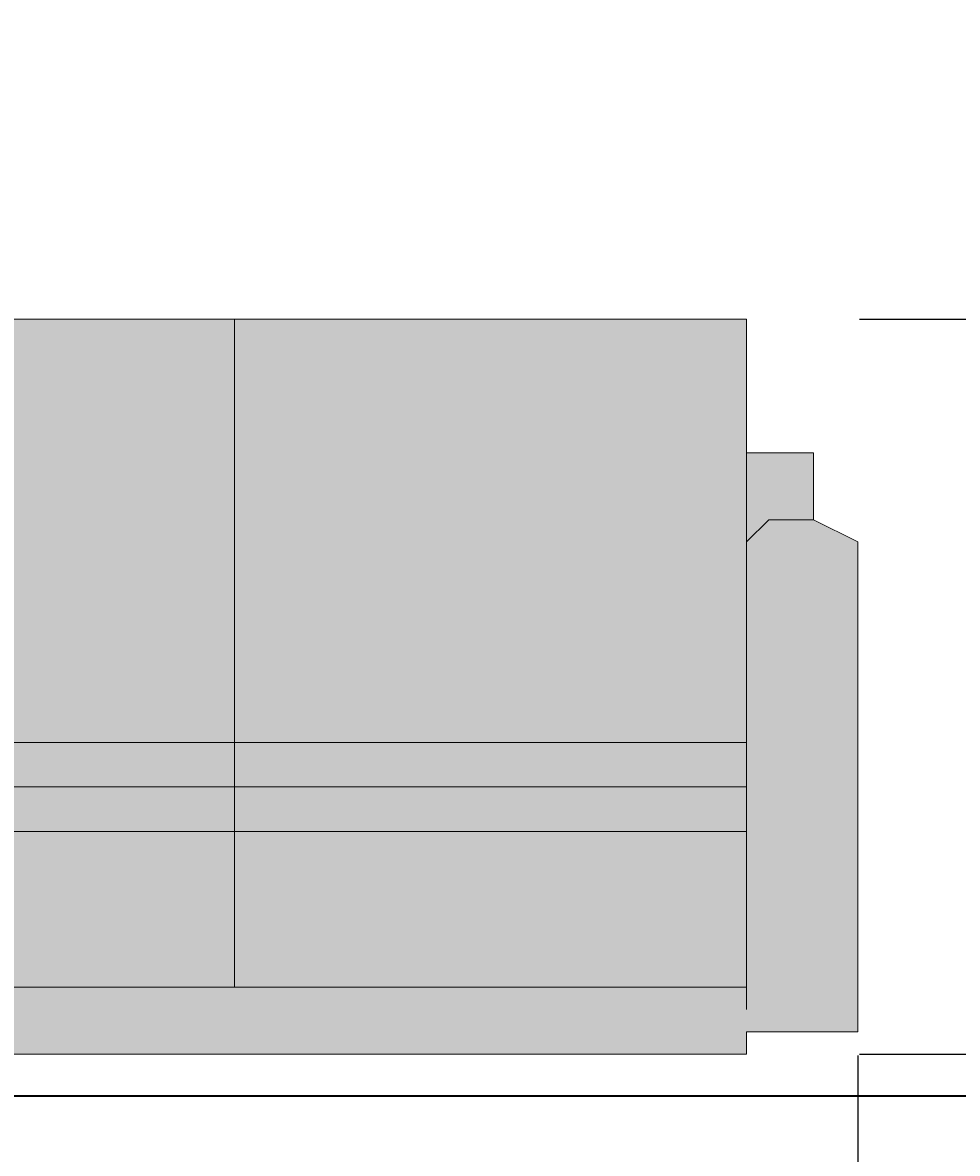
# Model space of a CAD drawing. Units: millimetres. Extents: x 27017497 to 27018854, y 7058029 to 7059154.
# Tile 35 of 91: x 27017714 to 27017750, y 7058297 to 7058341. Entities that reach past the tile are written whole.
import ezdxf

# ---------------------------------------------------------------- set-up
doc = ezdxf.new("R2010")
doc.units = ezdxf.units.MM
for name, color, linetype, lineweight in [('A-ANNO-DIMS', 2, 'Continuous', 18), ('A-FURN', 8, 'Continuous', 18), ('A-WALL', 7, 'Continuous', 35)]:
    doc.layers.add(name, color=color, linetype=linetype, lineweight=lineweight)
doc.layers.add('A-FURN-PATT', color=177, linetype='Continuous', lineweight=13, true_color=0x293189)
doc.styles.get("Standard").update_dxf_attribs({"font": 'arial.ttf'})
doc.dimstyles.get("Standard").update_dxf_attribs({"dimtxt": 0.18, "dimasz": 0.18, "dimexe": 0.18, "dimexo": 0.0625, "dimgap": 0.09, "dimtad": 0, "dimtih": 1, "dimtoh": 1, "dimdec": 4, "dimzin": 0, "dimdsep": 46, "dimtxsty": 'Standard', "dimcen": 0.09, "dimadec": 0, "dimazin": 0, "dimtfac": 1, "dimtdec": 4, "dimtofl": 0, "dimtmove": 0, "dimatfit": 3, "dimfxl": 1, "dimtolj": 1, "dimtzin": 0, "dimarcsym": 0})

# ---------------------------------------------------------------- blocks, each defined once
blk = doc.blocks.new('SOFA-LIVING-THREE-SEAT')
for p, q in [((63.532, 28.72), (4.351, 28.72)), ((43.515, 28.72), (43.515, 2.611)), ((63.532, 23.498), (63.532, 28.72)), ((63.532, 23.498), (63.532, 20.017)), ((66.142, 23.498), (63.532, 23.498)), ((66.142, 20.887), (66.142, 23.498)), ((64.402, 20.887), (63.532, 20.017)), ((66.142, 20.887), (64.402, 20.887)), ((67.883, 20.017), (66.142, 20.887)), ((63.532, 20.017), (63.532, 1.741)), ((67.883, 0.871), (67.883, 20.017)), ((63.532, 12.184), (4.351, 12.184)), ((63.532, 10.444), (4.351, 10.444)), ((63.532, 8.703), (4.351, 8.703)), ((4.351, 2.611), (63.532, 2.611)), ((63.532, 0), (63.532, 0.871)), ((63.532, 0.871), (67.883, 0.871)), ((4.351, 0), (63.532, 0))]:
    blk.add_line(p, q)
blk = doc.blocks.new('*D39')
at = {"layer": 'A-ANNO-DIMS', "color": 0, "lineweight": -2, "transparency": 16777216}
for p, q in [((27017678.38, 7058300.482), (27017678.38, 7058290.182)), ((27017746.263, 7058300.482), (27017746.263, 7058290.182)), ((27017678.56, 7058290.362), (27017710.973, 7058290.362)), ((27017746.083, 7058290.362), (27017713.67, 7058290.362))]:
    blk.add_line(p, q, dxfattribs=at)
at = {"layer": 'A-ANNO-DIMS', "color": 0, "transparency": 16777216}
for points in [[(27017678.56, 7058290.392), (27017678.56, 7058290.332), (27017678.38, 7058290.362)], [(27017746.083, 7058290.392), (27017746.083, 7058290.332), (27017746.263, 7058290.362)]]:
    blk.add_solid(points, dxfattribs=at)
at = {"layer": 'Defpoints', "color": 0, "transparency": 16777216}
for p in [(27017678.38, 7058300.544), (27017746.263, 7058300.544), (27017746.263, 7058290.362)]:
    blk.add_point(p, dxfattribs=at)
at = {"layer": 'A-ANNO-DIMS', "color": 0, "transparency": 16777216, "insert": (27017712.321, 7058290.362), "char_height": 0.18, "attachment_point": 5}
blk.add_mtext('\\A1;LIVING SOFA 68 TYP.', dxfattribs=at)
blk = doc.blocks.new('*D40')
at = {"layer": 'A-ANNO-DIMS', "color": 0, "lineweight": -2, "transparency": 16777216}
for p, q in [((27017746.325, 7058329.264), (27017756.625, 7058329.264)), ((27017756.445, 7058329.084), (27017756.445, 7058315.086)), ((27017756.445, 7058300.724), (27017756.445, 7058314.722)), ((27017746.325, 7058300.544), (27017756.625, 7058300.544))]:
    blk.add_line(p, q, dxfattribs=at)
at = {"layer": 'A-ANNO-DIMS', "color": 0, "transparency": 16777216}
for points in [[(27017756.415, 7058329.084), (27017756.475, 7058329.084), (27017756.445, 7058329.264)], [(27017756.415, 7058300.724), (27017756.475, 7058300.724), (27017756.445, 7058300.544)]]:
    blk.add_solid(points, dxfattribs=at)
at = {"layer": 'Defpoints', "color": 0, "transparency": 16777216}
for p in [(27017746.263, 7058329.264), (27017756.445, 7058329.264), (27017746.263, 7058300.544)]:
    blk.add_point(p, dxfattribs=at)
at = {"layer": 'A-ANNO-DIMS', "color": 0, "transparency": 16777216, "insert": (27017756.445, 7058314.904), "char_height": 0.18, "attachment_point": 5}
blk.add_mtext('\\A1;29 TYP.', dxfattribs=at)
blk = doc.blocks.new('*D48')
at = {"layer": 'A-ANNO-DIMS', "color": 0, "lineweight": -2, "transparency": 16777216}
for p, q in [((27018463.498, 7058622.912), (27017497.536, 7058622.912)), ((27017497.716, 7058622.732), (27017497.716, 7058357.753)), ((27017497.716, 7058092.41), (27017497.716, 7058357.389)), ((27018555.129, 7058092.23), (27017497.536, 7058092.23))]:
    blk.add_line(p, q, dxfattribs=at)
at = {"layer": 'A-ANNO-DIMS', "color": 0, "transparency": 16777216}
for points in [[(27017497.686, 7058622.732), (27017497.746, 7058622.732), (27017497.716, 7058622.912)], [(27017497.686, 7058092.41), (27017497.746, 7058092.41), (27017497.716, 7058092.23)]]:
    blk.add_solid(points, dxfattribs=at)
at = {"layer": 'Defpoints', "color": 0, "transparency": 16777216}
for p in [(27018463.561, 7058622.912), (27017497.716, 7058092.23), (27018555.192, 7058092.23)]:
    blk.add_point(p, dxfattribs=at)
at = {"layer": 'A-ANNO-DIMS', "color": 0, "transparency": 16777216, "insert": (27017497.716, 7058357.571), "char_height": 0.18, "attachment_point": 5}
blk.add_mtext('\\A1;530.7', dxfattribs=at)

msp = doc.modelspace()

# ---------------------------------------------------------------- hatches: boundary and pattern name
at = {"layer": 'A-FURN-PATT'}
h = msp.add_hatch(color=256, dxfattribs=at)
h.dxf.hatch_style = 1
h.paths.add_polyline_path([(27017702.748, 7058329.264), (27017682.731, 7058329.264), (27017682.731, 7058324.042), (27017682.731, 7058320.561), (27017682.731, 7058312.728), (27017702.748, 7058312.728)])
h.paths.add_polyline_path([(27017721.895, 7058329.264), (27017702.748, 7058329.264), (27017702.748, 7058312.728), (27017721.895, 7058312.728)])
h.paths.add_polyline_path([(27017741.912, 7058320.561), (27017741.912, 7058324.042), (27017741.912, 7058329.264), (27017721.895, 7058329.264), (27017721.895, 7058312.728), (27017741.912, 7058312.728)])
h.paths.add_polyline_path([(27017682.731, 7058320.561), (27017681.861, 7058321.431), (27017680.121, 7058321.431), (27017678.38, 7058320.561), (27017678.38, 7058301.415), (27017682.731, 7058301.415), (27017682.731, 7058300.544), (27017741.912, 7058300.544), (27017741.912, 7058301.415), (27017746.263, 7058301.415), (27017746.263, 7058320.561), (27017744.522, 7058321.431), (27017742.782, 7058321.431), (27017741.912, 7058320.561), (27017741.912, 7058303.155), (27017682.731, 7058303.155)])
h.paths.add_polyline_path([(27017741.912, 7058309.247), (27017721.895, 7058309.247), (27017721.895, 7058303.155), (27017741.912, 7058303.155)], flags=17)
h.paths.add_polyline_path([(27017721.895, 7058309.247), (27017702.748, 7058309.247), (27017702.748, 7058303.155), (27017721.895, 7058303.155)], flags=17)
h.paths.add_polyline_path([(27017702.748, 7058309.247), (27017682.731, 7058309.247), (27017682.731, 7058303.155), (27017702.748, 7058303.155)], flags=17)
h.paths.add_polyline_path([(27017702.748, 7058312.728), (27017682.731, 7058312.728), (27017682.731, 7058310.988), (27017702.748, 7058310.988)], flags=17)
h.paths.add_polyline_path([(27017721.895, 7058312.728), (27017702.748, 7058312.728), (27017702.748, 7058310.988), (27017721.895, 7058310.988)], flags=17)
h.paths.add_polyline_path([(27017741.912, 7058312.728), (27017721.895, 7058312.728), (27017721.895, 7058310.988), (27017741.912, 7058310.988)], flags=17)
h.paths.add_polyline_path([(27017741.912, 7058310.988), (27017721.895, 7058310.988), (27017721.895, 7058309.247), (27017741.912, 7058309.247)], flags=17)
h.paths.add_polyline_path([(27017721.895, 7058310.988), (27017702.748, 7058310.988), (27017702.748, 7058309.247), (27017721.895, 7058309.247)], flags=17)
h.paths.add_polyline_path([(27017702.748, 7058310.988), (27017682.731, 7058310.988), (27017682.731, 7058309.247), (27017702.748, 7058309.247)], flags=17)
h.paths.add_polyline_path([(27017744.522, 7058324.042), (27017741.912, 7058324.042), (27017741.912, 7058320.561), (27017742.782, 7058321.431), (27017744.522, 7058321.431)])
h.paths.add_polyline_path([(27017682.731, 7058324.042), (27017680.121, 7058324.042), (27017680.121, 7058321.431), (27017681.861, 7058321.431), (27017682.731, 7058320.561)])

# ---------------------------------------------------------------- linework, layer by layer
at = {"layer": 'A-WALL'}
for p, q in [((27017641.166, 7058298.912), (27017743.666, 7058298.912)), ((27017743.666, 7058298.912), (27017758.779, 7058298.912))]:
    msp.add_line(p, q, dxfattribs=at)

# ---------------------------------------------------------------- block references
at = {"layer": 'A-FURN'}
msp.add_blockref('SOFA-LIVING-THREE-SEAT', (27017678.38, 7058300.544), dxfattribs=at)

# ---------------------------------------------------------------- dimensions: what is measured, and where the dimension line sits
at = {"layer": 'A-ANNO-DIMS'}
dim = msp.add_linear_dim(base=(27017497.716, 7058092.23), p1=(27018463.561, 7058622.912), p2=(27018555.192, 7058092.23), angle=90, dimstyle='Standard', override={"dimdec": 1, "dimlfac": 1, "dimrnd": 0, "dimzin": 0, "dimdsep": 46, "dimlunit": 2}, dxfattribs=at)
dim.commit()
dim.dimension.update_dxf_attribs({"geometry": '*D48', "text_midpoint": (27017497.716, 7058357.571)})
dim = msp.add_linear_dim(base=(27017756.445, 7058329.264), p1=(27017746.263, 7058300.544), p2=(27017746.263, 7058329.264), angle=90, text='<> TYP.', dimstyle='Standard', override={"dimdec": 0, "dimlfac": 1, "dimrnd": 0, "dimzin": 0, "dimdsep": 46, "dimlunit": 2}, dxfattribs=at)
dim.commit()
dim.dimension.update_dxf_attribs({"geometry": '*D40', "text_midpoint": (27017756.445, 7058314.904)})
dim = msp.add_linear_dim(base=(27017746.263, 7058290.362), p1=(27017678.38, 7058300.544), p2=(27017746.263, 7058300.544), text='LIVING SOFA <> TYP.', dimstyle='Standard', override={"dimdec": 0, "dimlfac": 1, "dimrnd": 0, "dimzin": 0, "dimdsep": 46, "dimlunit": 2}, dxfattribs=at)
dim.commit()
dim.dimension.update_dxf_attribs({"geometry": '*D39', "text_midpoint": (27017712.321, 7058290.362)})

doc.saveas('drawing.dxf')
